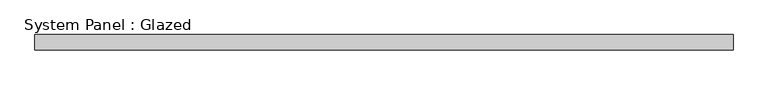
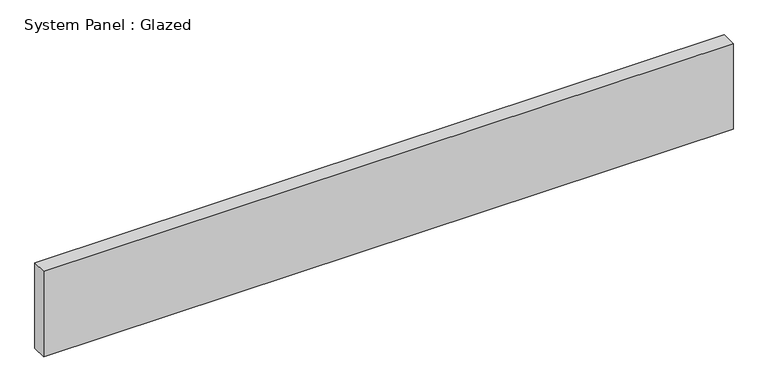
"""IFC4 building model written with IfcOpenShell, lengths in millimetres: plate geometry, System Panel : Glazed."""

from ifc_helpers import new_model, si_unit, origin, origin_with_axes, place, context, project, spatial, polyline, outline, extrude, source, transform, mapped, element, save


def system_panel_glazed_325d72d1(model_context):
    return source(origin(), model_context, "Body", "SweptSolid", [
        extrude(outline(polyline([(571.7712628, 24.5), (-571.7712628, 24.5), (-571.7712628, 49.5), (571.7712628, 49.5), (571.7712628, 24.5)])), origin_with_axes(), (0.0, 0.0, 1.0), 150.0429688),
    ])


if __name__ == "__main__":
    model = new_model("IFC4")
    model_context = context("Model", 3, world=origin())
    ifc_project = project(units=[si_unit("LENGTHUNIT", "METRE", prefix="MILLI")], contexts=[model_context])
    site = spatial("IfcSite", under=ifc_project)
    building = spatial("IfcBuilding", under=site)
    placement = place(None, origin())
    system_panel_glazed_shape = system_panel_glazed_325d72d1(model_context)
    element("IfcPlate", 1, ObjectType="System Panel : Glazed", at=placement, inside=building, context=model_context, shape_type="MappedRepresentation", body=[
        mapped(system_panel_glazed_shape, transform((0.0, 0.0, 0.0), x_axis=(1.0, 0.0, 0.0), y_axis=(0.0, 1.0, 0.0), z_axis=(0.0, 0.0, 1.0))),
    ])
    save(model, "model.ifc")

# Revit data of these elements
# Type "System Panel : Glazed"
#   Keynote = "H11"
#   Construction Type Id = "GSP4R"
#   Analytic Construction = "1/8 in Pilkington single glazing"
#   Visual Light Transmittance = 0.9
#   Solar Heat Gain Coefficient = 0.86
#   Heat Transfer Coefficient (U) = 6.7069 W/(m²·K)
#   Define Thermal Properties by = 1
# Element 1 (IfcPlate, "System Panel : Glazed")
#   Materials on its faces: "Glass"
# Materials
#   "Glass": class "Glass", colour RGB 0 128 192, transparency 0.9, Description = "Soda Lime Glass", Cost = 0
